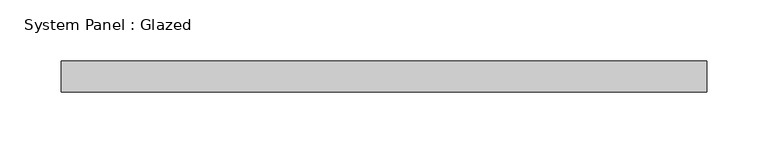
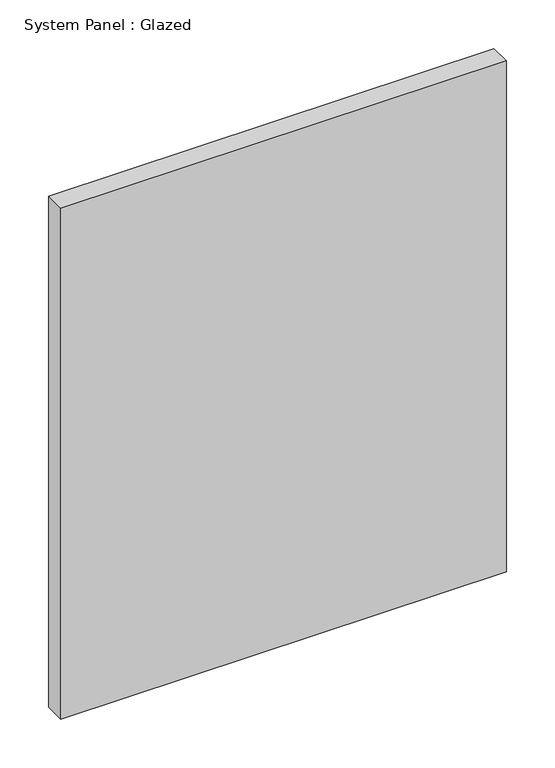
"""IFC4 building model written with IfcOpenShell, lengths in millimetres: plate geometry, System Panel : Glazed."""

from ifc_helpers import new_model, si_unit, origin, origin_with_axes, place, context, project, spatial, polyline, outline, extrude, source, transform, mapped, element, save


def system_panel_glazed_32595814(model_context):
    return source(origin(), model_context, "Body", "SweptSolid", [
        extrude(outline(polyline([(264.5833333, 19.05), (-264.5833333, 19.05), (-264.5833333, 44.45), (264.5833333, 44.45), (264.5833333, 19.05)])), origin_with_axes(), (0.0, 0.0, 1.0), 641.35),
    ])


if __name__ == "__main__":
    model = new_model("IFC4")
    model_context = context("Model", 3, world=origin())
    ifc_project = project(units=[si_unit("LENGTHUNIT", "METRE", prefix="MILLI")], contexts=[model_context])
    site = spatial("IfcSite", under=ifc_project)
    building = spatial("IfcBuilding", under=site)
    placement = place(None, origin())
    system_panel_glazed_shape = system_panel_glazed_32595814(model_context)
    element("IfcPlate", 1, ObjectType="System Panel : Glazed", at=placement, inside=building, context=model_context, shape_type="MappedRepresentation", body=[
        mapped(system_panel_glazed_shape, transform((0.0, 0.0, 0.0), x_axis=(1.0, 0.0, 0.0), y_axis=(0.0, 1.0, 0.0), z_axis=(0.0, 0.0, 1.0))),
    ])
    save(model, "model.ifc")

# Revit data of these elements
# Type "System Panel : Glazed"
#   Construction Type Id = "GSP4R"
#   Analytic Construction = "1/8 in Pilkington single glazing"
#   Visual Light Transmittance = 0.9
#   Solar Heat Gain Coefficient = 0.86
#   Heat Transfer Coefficient (U) = 1.18115 BTU/(h·ft²·°F)
#   Define Thermal Properties by = 1
# Element 1 (IfcPlate, "System Panel : Glazed")
#   Materials on its faces: "Glass"
# Materials
#   "Glass": class "Glass", colour RGB 0 128 192, transparency 0.75, Description = "Soda Lime Glass", Cost = 0
